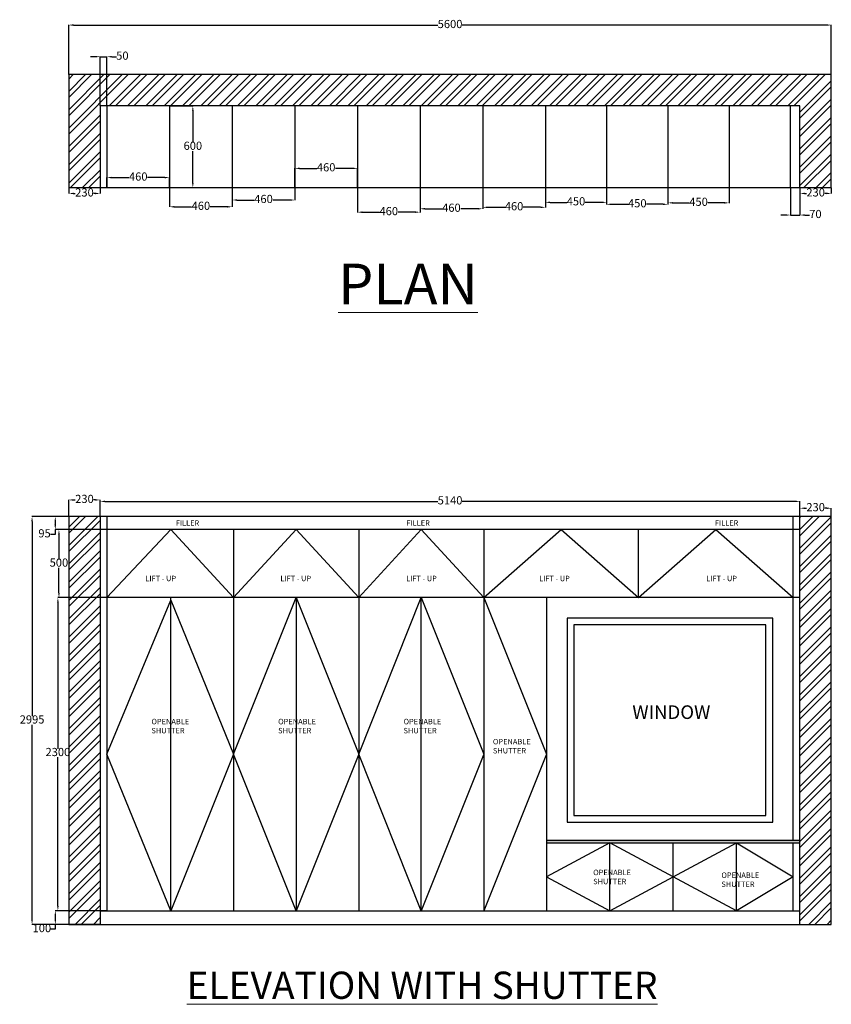
# Model space of a CAD drawing. Units: millimetres. Extents: x 1304 to 14372, y 283 to 7516.
# Tile 4 of 4: x 8411 to 14372, y 283 to 7516. Entities that reach past the tile are written whole.
import ezdxf

# ---------------------------------------------------------------- set-up
doc = ezdxf.new("R2010")
doc.units = ezdxf.units.MM
doc.layers.get('Defpoints').update_dxf_attribs({"color": 2})
for name, color, linetype, lineweight in [('A-ANNO-DIMS', 2, 'Continuous', 18), ('A-ANNO-TEXT', 3, 'Continuous', 18), ('A-FURN', 7, 'Continuous', 25), ('A-FURN-PATT', 8, 'Continuous', 13)]:
    doc.layers.add(name, color=color, linetype=linetype, lineweight=lineweight)
doc.styles.get("Standard").update_dxf_attribs({"font": 'arial.ttf'})
doc.dimstyles.new('ISO-25', dxfattribs={"dimtxt": 60, "dimasz": 35, "dimexe": 1.25, "dimexo": 0.625, "dimtad": 0, "dimtih": 1, "dimtoh": 1, "dimtxsty": 'Standard', "dimcen": 2.5, "dimclrd": 1, "dimclre": 3, "dimadec": 0, "dimazin": 0, "dimtfac": 1, "dimtmove": 0, "dimatfit": 3, "dimfxl": 1, "dimarcsym": 0})

# ---------------------------------------------------------------- blocks, each defined once
blk = doc.blocks.new('*D46')
at = {"layer": 'A-ANNO-DIMS', "color": 0, "lineweight": -2, "transparency": 16777216}
for p, q in [((8771.4, 3865.3), (8500.9, 3865.3)), ((8502.2, 3830.3), (8502.2, 2399)), ((8502.2, 905.3), (8502.2, 2336.5)), ((8771.4, 870.3), (8500.9, 870.3))]:
    blk.add_line(p, q, dxfattribs=at)
at = {"layer": 'A-ANNO-DIMS', "color": 0, "transparency": 16777216}
for points in [[(8496.3, 3830.3), (8508, 3830.3), (8502.2, 3865.3)], [(8496.3, 905.3), (8508, 905.3), (8502.2, 870.3)]]:
    blk.add_solid(points, dxfattribs=at)
at = {"layer": 'Defpoints', "color": 0, "transparency": 16777216}
for p in [(8772, 3865.3), (8502.2, 870.3), (8772, 870.3)]:
    blk.add_point(p, dxfattribs=at)
at = {"layer": 'A-ANNO-DIMS', "color": 0, "transparency": 16777216, "insert": (8502.2, 2367.8), "char_height": 60, "attachment_point": 5}
blk.add_mtext('2995', dxfattribs=at)
blk = doc.blocks.new('*D47')
at = {"layer": 'A-ANNO-DIMS', "color": 0, "lineweight": -2, "transparency": 16777216}
for p, q in [((9001.4, 3865.3), (8671.3, 3865.3)), ((9001.4, 3770.3), (8671.3, 3770.3)), ((8672.5, 3830.3), (8672.5, 3805.3)), ((8672.5, 3770.3), (8672.5, 3735.3)), ((8672.5, 3735.3), (8637.5, 3735.3))]:
    blk.add_line(p, q, dxfattribs=at)
at = {"layer": 'A-ANNO-DIMS', "color": 0, "transparency": 16777216}
for points in [[(8666.7, 3830.3), (8678.4, 3830.3), (8672.5, 3865.3)], [(8666.7, 3805.3), (8678.4, 3805.3), (8672.5, 3770.3)]]:
    blk.add_solid(points, dxfattribs=at)
at = {"layer": 'Defpoints', "color": 0, "transparency": 16777216}
for p in [(9002, 3865.3), (8672.5, 3770.3), (9002, 3770.3)]:
    blk.add_point(p, dxfattribs=at)
at = {"layer": 'A-ANNO-DIMS', "color": 0, "transparency": 16777216, "insert": (8593.7, 3735.3), "char_height": 60, "attachment_point": 5}
blk.add_mtext('95', dxfattribs=at)
blk = doc.blocks.new('*D48')
at = {"layer": 'A-ANNO-DIMS', "color": 0, "lineweight": -2, "transparency": 16777216}
for p, q in [((9051.4, 3770.3), (8698.2, 3770.3)), ((8699.5, 3735.3), (8699.5, 3551.5)), ((8699.5, 3305.3), (8699.5, 3489)), ((9051.4, 3270.3), (8698.2, 3270.3))]:
    blk.add_line(p, q, dxfattribs=at)
at = {"layer": 'A-ANNO-DIMS', "color": 0, "transparency": 16777216}
for points in [[(8693.6, 3735.3), (8705.3, 3735.3), (8699.5, 3770.3)], [(8693.6, 3305.3), (8705.3, 3305.3), (8699.5, 3270.3)]]:
    blk.add_solid(points, dxfattribs=at)
at = {"layer": 'Defpoints', "color": 0, "transparency": 16777216}
for p in [(9052, 3770.3), (8699.5, 3270.3), (9052, 3270.3)]:
    blk.add_point(p, dxfattribs=at)
at = {"layer": 'A-ANNO-DIMS', "color": 0, "transparency": 16777216, "insert": (8699.5, 3520.3), "char_height": 60, "attachment_point": 5}
blk.add_mtext('500', dxfattribs=at)
blk = doc.blocks.new('*D49')
at = {"layer": 'A-ANNO-DIMS', "color": 0, "lineweight": -2, "transparency": 16777216}
for p, q in [((9001.4, 970.3), (8671.7, 970.3)), ((9001.4, 870.3), (8671.7, 870.3)), ((8673, 935.3), (8673, 905.3)), ((8673, 870.3), (8673, 835.3)), ((8673, 835.3), (8638, 835.3))]:
    blk.add_line(p, q, dxfattribs=at)
at = {"layer": 'A-ANNO-DIMS', "color": 0, "transparency": 16777216}
for points in [[(8667.1, 935.3), (8678.8, 935.3), (8673, 970.3)], [(8667.1, 905.3), (8678.8, 905.3), (8673, 870.3)]]:
    blk.add_solid(points, dxfattribs=at)
at = {"layer": 'Defpoints', "color": 0, "transparency": 16777216}
for p in [(9002, 970.3), (8673, 870.3), (9002, 870.3)]:
    blk.add_point(p, dxfattribs=at)
at = {"layer": 'A-ANNO-DIMS', "color": 0, "transparency": 16777216, "insert": (8574, 835.3), "char_height": 60, "attachment_point": 5}
blk.add_mtext('100', dxfattribs=at)
blk = doc.blocks.new('*D50')
at = {"layer": 'A-ANNO-DIMS', "color": 0, "lineweight": -2, "transparency": 16777216}
for p, q in [((9051.4, 3270.3), (8690.6, 3270.3)), ((8691.9, 3235.3), (8691.9, 2160)), ((8691.9, 1005.3), (8691.9, 2097.5)), ((9051.4, 970.3), (8690.6, 970.3))]:
    blk.add_line(p, q, dxfattribs=at)
at = {"layer": 'A-ANNO-DIMS', "color": 0, "transparency": 16777216}
for points in [[(8686.1, 3235.3), (8697.7, 3235.3), (8691.9, 3270.3)], [(8686.1, 1005.3), (8697.7, 1005.3), (8691.9, 970.3)]]:
    blk.add_solid(points, dxfattribs=at)
at = {"layer": 'Defpoints', "color": 0, "transparency": 16777216}
for p in [(9052, 3270.3), (8691.9, 970.3), (9052, 970.3)]:
    blk.add_point(p, dxfattribs=at)
at = {"layer": 'A-ANNO-DIMS', "color": 0, "transparency": 16777216, "insert": (8691.9, 2128.8), "char_height": 60, "attachment_point": 5}
blk.add_mtext('2300', dxfattribs=at)
blk = doc.blocks.new('*D51')
at = {"layer": 'A-ANNO-DIMS', "color": 0, "lineweight": -2, "transparency": 16777216}
for p, q in [((8772, 3865.9), (8772, 3989.4)), ((8807, 3988.1), (8819.7, 3988.1)), ((8967, 3988.1), (8954.3, 3988.1)), ((9002, 3865.9), (9002, 3989.4))]:
    blk.add_line(p, q, dxfattribs=at)
at = {"layer": 'A-ANNO-DIMS', "color": 0, "transparency": 16777216}
for points in [[(8807, 3993.9), (8807, 3982.3), (8772, 3988.1)], [(8967, 3993.9), (8967, 3982.3), (9002, 3988.1)]]:
    blk.add_solid(points, dxfattribs=at)
at = {"layer": 'Defpoints', "color": 0, "transparency": 16777216}
for p in [(9002, 3988.1), (8772, 3865.3), (9002, 3865.3)]:
    blk.add_point(p, dxfattribs=at)
at = {"layer": 'A-ANNO-DIMS', "color": 0, "transparency": 16777216, "insert": (8887, 3988.1), "char_height": 60, "attachment_point": 5}
blk.add_mtext('230', dxfattribs=at)
blk = doc.blocks.new('*D52')
at = {"layer": 'A-ANNO-DIMS', "color": 0, "lineweight": -2, "transparency": 16777216}
for p, q in [((14142, 3865.9), (14142, 3928.7)), ((14177, 3927.4), (14189.7, 3927.4)), ((14337, 3927.4), (14324.3, 3927.4)), ((14372, 3865.9), (14372, 3928.7))]:
    blk.add_line(p, q, dxfattribs=at)
at = {"layer": 'A-ANNO-DIMS', "color": 0, "transparency": 16777216}
for points in [[(14177, 3933.2), (14177, 3921.6), (14142, 3927.4)], [(14337, 3933.2), (14337, 3921.6), (14372, 3927.4)]]:
    blk.add_solid(points, dxfattribs=at)
at = {"layer": 'Defpoints', "color": 0, "transparency": 16777216}
for p in [(14372, 3927.4), (14142, 3865.3), (14372, 3865.3)]:
    blk.add_point(p, dxfattribs=at)
at = {"layer": 'A-ANNO-DIMS', "color": 0, "transparency": 16777216, "insert": (14257, 3927.4), "char_height": 60, "attachment_point": 5}
blk.add_mtext('230', dxfattribs=at)
blk = doc.blocks.new('*D53')
at = {"layer": 'A-ANNO-DIMS', "color": 0, "lineweight": -2, "transparency": 16777216}
for p, q in [((9002, 3865.9), (9002, 3978.7)), ((14142, 3865.9), (14142, 3978.7)), ((9037, 3977.4), (11481.9, 3977.4)), ((14107, 3977.4), (11662.1, 3977.4))]:
    blk.add_line(p, q, dxfattribs=at)
at = {"layer": 'A-ANNO-DIMS', "color": 0, "transparency": 16777216}
for points in [[(9037, 3983.2), (9037, 3971.6), (9002, 3977.4)], [(14107, 3983.2), (14107, 3971.6), (14142, 3977.4)]]:
    blk.add_solid(points, dxfattribs=at)
at = {"layer": 'Defpoints', "color": 0, "transparency": 16777216}
for p in [(14142, 3977.4), (9002, 3865.3), (14142, 3865.3)]:
    blk.add_point(p, dxfattribs=at)
at = {"layer": 'A-ANNO-DIMS', "color": 0, "transparency": 16777216, "insert": (11572, 3977.4), "char_height": 60, "attachment_point": 5}
blk.add_mtext('5140', dxfattribs=at)
blk = doc.blocks.new('*D54')
at = {"layer": 'A-ANNO-DIMS', "color": 0, "lineweight": -2, "transparency": 16777216}
for p, q in [((8772, 6281.6), (8772, 6238)), ((8807, 6239.3), (8819.7, 6239.3)), ((8967, 6239.3), (8954.3, 6239.3)), ((9002, 6281.6), (9002, 6238))]:
    blk.add_line(p, q, dxfattribs=at)
at = {"layer": 'A-ANNO-DIMS', "color": 0, "transparency": 16777216}
for points in [[(8807, 6245.1), (8807, 6233.4), (8772, 6239.3)], [(8967, 6245.1), (8967, 6233.4), (9002, 6239.3)]]:
    blk.add_solid(points, dxfattribs=at)
at = {"layer": 'Defpoints', "color": 0, "transparency": 16777216}
for p in [(8772, 6282.2), (9002, 6282.2), (9002, 6239.3)]:
    blk.add_point(p, dxfattribs=at)
at = {"layer": 'A-ANNO-DIMS', "color": 0, "transparency": 16777216, "insert": (8887, 6239.3), "char_height": 60, "attachment_point": 5}
blk.add_mtext('230', dxfattribs=at)
blk = doc.blocks.new('*D55')
at = {"layer": 'A-ANNO-DIMS', "color": 0, "lineweight": -2, "transparency": 16777216}
for p, q in [((8967, 7244), (8932, 7244)), ((9002, 6882.8), (9002, 7245.2)), ((9002, 7244), (9052, 7244)), ((9052, 6882.8), (9052, 7245.2)), ((9087, 7244), (9122, 7244))]:
    blk.add_line(p, q, dxfattribs=at)
at = {"layer": 'A-ANNO-DIMS', "color": 0, "transparency": 16777216}
for points in [[(8967, 7249.8), (8967, 7238.2), (9002, 7244)], [(9087, 7249.8), (9087, 7238.2), (9052, 7244)]]:
    blk.add_solid(points, dxfattribs=at)
at = {"layer": 'Defpoints', "color": 0, "transparency": 16777216}
for p in [(9052, 7244), (9002, 6882.2), (9052, 6882.2)]:
    blk.add_point(p, dxfattribs=at)
at = {"layer": 'A-ANNO-DIMS', "color": 0, "transparency": 16777216, "insert": (9165.5, 7244), "char_height": 60, "attachment_point": 5}
blk.add_mtext('50', dxfattribs=at)
blk = doc.blocks.new('*D56')
at = {"layer": 'A-ANNO-DIMS', "color": 0, "lineweight": -2, "transparency": 16777216}
for p, q in [((9052, 6282.8), (9052, 6357.4)), ((9087, 6356.1), (9214, 6356.1)), ((9477, 6356.1), (9350, 6356.1)), ((9512, 6282.8), (9512, 6357.4))]:
    blk.add_line(p, q, dxfattribs=at)
at = {"layer": 'A-ANNO-DIMS', "color": 0, "transparency": 16777216}
for points in [[(9087, 6361.9), (9087, 6350.3), (9052, 6356.1)], [(9477, 6361.9), (9477, 6350.3), (9512, 6356.1)]]:
    blk.add_solid(points, dxfattribs=at)
at = {"layer": 'Defpoints', "color": 0, "transparency": 16777216}
for p in [(9512, 6356.1), (9052, 6282.2), (9512, 6282.2)]:
    blk.add_point(p, dxfattribs=at)
at = {"layer": 'A-ANNO-DIMS', "color": 0, "transparency": 16777216, "insert": (9282, 6356.1), "char_height": 60, "attachment_point": 5}
blk.add_mtext('460', dxfattribs=at)
blk = doc.blocks.new('*D57')
at = {"layer": 'A-ANNO-DIMS', "color": 0, "lineweight": -2, "transparency": 16777216}
for p, q in [((9512, 6281.6), (9512, 6140.1)), ((9972, 6281.6), (9972, 6140.1)), ((9547, 6141.3), (9674, 6141.3)), ((9937, 6141.3), (9810, 6141.3))]:
    blk.add_line(p, q, dxfattribs=at)
at = {"layer": 'A-ANNO-DIMS', "color": 0, "transparency": 16777216}
for points in [[(9547, 6147.2), (9547, 6135.5), (9512, 6141.3)], [(9937, 6147.2), (9937, 6135.5), (9972, 6141.3)]]:
    blk.add_solid(points, dxfattribs=at)
at = {"layer": 'Defpoints', "color": 0, "transparency": 16777216}
for p in [(9512, 6282.2), (9972, 6282.2), (9972, 6141.3)]:
    blk.add_point(p, dxfattribs=at)
at = {"layer": 'A-ANNO-DIMS', "color": 0, "transparency": 16777216, "insert": (9742, 6141.3), "char_height": 60, "attachment_point": 5}
blk.add_mtext('460', dxfattribs=at)
blk = doc.blocks.new('*D58')
at = {"layer": 'A-ANNO-DIMS', "color": 0, "lineweight": -2, "transparency": 16777216}
for p, q in [((9972, 6281.6), (9972, 6190.2)), ((10432, 6281.6), (10432, 6190.2)), ((10007, 6191.4), (10134, 6191.4)), ((10397, 6191.4), (10270, 6191.4))]:
    blk.add_line(p, q, dxfattribs=at)
at = {"layer": 'A-ANNO-DIMS', "color": 0, "transparency": 16777216}
for points in [[(10007, 6197.2), (10007, 6185.6), (9972, 6191.4)], [(10397, 6197.2), (10397, 6185.6), (10432, 6191.4)]]:
    blk.add_solid(points, dxfattribs=at)
at = {"layer": 'Defpoints', "color": 0, "transparency": 16777216}
for p in [(9972, 6282.2), (10432, 6282.2), (10432, 6191.4)]:
    blk.add_point(p, dxfattribs=at)
at = {"layer": 'A-ANNO-DIMS', "color": 0, "transparency": 16777216, "insert": (10202, 6191.4), "char_height": 60, "attachment_point": 5}
blk.add_mtext('460', dxfattribs=at)
blk = doc.blocks.new('*D59')
at = {"layer": 'A-ANNO-DIMS', "color": 0, "lineweight": -2, "transparency": 16777216}
for p, q in [((10432, 6282.8), (10432, 6425.1)), ((10467, 6423.9), (10594, 6423.9)), ((10857, 6423.9), (10730, 6423.9)), ((10892, 6282.8), (10892, 6425.1))]:
    blk.add_line(p, q, dxfattribs=at)
at = {"layer": 'A-ANNO-DIMS', "color": 0, "transparency": 16777216}
for points in [[(10467, 6429.7), (10467, 6418), (10432, 6423.9)], [(10857, 6429.7), (10857, 6418), (10892, 6423.9)]]:
    blk.add_solid(points, dxfattribs=at)
at = {"layer": 'Defpoints', "color": 0, "transparency": 16777216}
for p in [(10892, 6423.9), (10432, 6282.2), (10892, 6282.2)]:
    blk.add_point(p, dxfattribs=at)
at = {"layer": 'A-ANNO-DIMS', "color": 0, "transparency": 16777216, "insert": (10662, 6423.9), "char_height": 60, "attachment_point": 5}
blk.add_mtext('460', dxfattribs=at)
blk = doc.blocks.new('*D60')
at = {"layer": 'A-ANNO-DIMS', "color": 0, "lineweight": -2, "transparency": 16777216}
for p, q in [((10892, 6281.6), (10892, 6100.7)), ((11352, 6281.6), (11352, 6100.7)), ((10927, 6102), (11054, 6102)), ((11317, 6102), (11190, 6102))]:
    blk.add_line(p, q, dxfattribs=at)
at = {"layer": 'A-ANNO-DIMS', "color": 0, "transparency": 16777216}
for points in [[(10927, 6107.8), (10927, 6096.2), (10892, 6102)], [(11317, 6107.8), (11317, 6096.2), (11352, 6102)]]:
    blk.add_solid(points, dxfattribs=at)
at = {"layer": 'Defpoints', "color": 0, "transparency": 16777216}
for p in [(10892, 6282.2), (11352, 6282.2), (11352, 6102)]:
    blk.add_point(p, dxfattribs=at)
at = {"layer": 'A-ANNO-DIMS', "color": 0, "transparency": 16777216, "insert": (11122, 6102), "char_height": 60, "attachment_point": 5}
blk.add_mtext('460', dxfattribs=at)
blk = doc.blocks.new('*D61')
at = {"layer": 'A-ANNO-DIMS', "color": 0, "lineweight": -2, "transparency": 16777216}
for p, q in [((11352, 6281.6), (11352, 6125.8)), ((11812, 6281.6), (11812, 6125.8)), ((11387, 6127), (11514, 6127)), ((11777, 6127), (11650, 6127))]:
    blk.add_line(p, q, dxfattribs=at)
at = {"layer": 'A-ANNO-DIMS', "color": 0, "transparency": 16777216}
for points in [[(11387, 6132.9), (11387, 6121.2), (11352, 6127)], [(11777, 6132.9), (11777, 6121.2), (11812, 6127)]]:
    blk.add_solid(points, dxfattribs=at)
at = {"layer": 'Defpoints', "color": 0, "transparency": 16777216}
for p in [(11352, 6282.2), (11812, 6282.2), (11812, 6127)]:
    blk.add_point(p, dxfattribs=at)
at = {"layer": 'A-ANNO-DIMS', "color": 0, "transparency": 16777216, "insert": (11582, 6127), "char_height": 60, "attachment_point": 5}
blk.add_mtext('460', dxfattribs=at)
blk = doc.blocks.new('*D62')
at = {"layer": 'A-ANNO-DIMS', "color": 0, "lineweight": -2, "transparency": 16777216}
for p, q in [((11812, 6281.6), (11812, 6136.5)), ((12272, 6281.6), (12272, 6136.5)), ((11847, 6137.8), (11974, 6137.8)), ((12237, 6137.8), (12110, 6137.8))]:
    blk.add_line(p, q, dxfattribs=at)
at = {"layer": 'A-ANNO-DIMS', "color": 0, "transparency": 16777216}
for points in [[(11847, 6143.6), (11847, 6131.9), (11812, 6137.8)], [(12237, 6143.6), (12237, 6131.9), (12272, 6137.8)]]:
    blk.add_solid(points, dxfattribs=at)
at = {"layer": 'Defpoints', "color": 0, "transparency": 16777216}
for p in [(11812, 6282.2), (12272, 6282.2), (12272, 6137.8)]:
    blk.add_point(p, dxfattribs=at)
at = {"layer": 'A-ANNO-DIMS', "color": 0, "transparency": 16777216, "insert": (12042, 6137.8), "char_height": 60, "attachment_point": 5}
blk.add_mtext('460', dxfattribs=at)
blk = doc.blocks.new('*D63')
at = {"layer": 'A-ANNO-DIMS', "color": 0, "lineweight": -2, "transparency": 16777216}
for p, q in [((12272, 6281.6), (12272, 6172.9)), ((12722, 6281.6), (12722, 6172.9)), ((12307, 6174.1), (12429, 6174.1)), ((12687, 6174.1), (12565, 6174.1))]:
    blk.add_line(p, q, dxfattribs=at)
at = {"layer": 'A-ANNO-DIMS', "color": 0, "transparency": 16777216}
for points in [[(12307, 6180), (12307, 6168.3), (12272, 6174.1)], [(12687, 6180), (12687, 6168.3), (12722, 6174.1)]]:
    blk.add_solid(points, dxfattribs=at)
at = {"layer": 'Defpoints', "color": 0, "transparency": 16777216}
for p in [(12272, 6282.2), (12722, 6282.2), (12722, 6174.1)]:
    blk.add_point(p, dxfattribs=at)
at = {"layer": 'A-ANNO-DIMS', "color": 0, "transparency": 16777216, "insert": (12497, 6174.1), "char_height": 60, "attachment_point": 5}
blk.add_mtext('450', dxfattribs=at)
blk = doc.blocks.new('*D64')
at = {"layer": 'A-ANNO-DIMS', "color": 0, "lineweight": -2, "transparency": 16777216}
for p, q in [((12722, 6281.6), (12722, 6158.5)), ((13172, 6281.6), (13172, 6158.5)), ((12757, 6159.8), (12879, 6159.8)), ((13137, 6159.8), (13015, 6159.8))]:
    blk.add_line(p, q, dxfattribs=at)
at = {"layer": 'A-ANNO-DIMS', "color": 0, "transparency": 16777216}
for points in [[(12757, 6165.6), (12757, 6153.9), (12722, 6159.8)], [(13137, 6165.6), (13137, 6153.9), (13172, 6159.8)]]:
    blk.add_solid(points, dxfattribs=at)
at = {"layer": 'Defpoints', "color": 0, "transparency": 16777216}
for p in [(12722, 6282.2), (13172, 6282.2), (13172, 6159.8)]:
    blk.add_point(p, dxfattribs=at)
at = {"layer": 'A-ANNO-DIMS', "color": 0, "transparency": 16777216, "insert": (12947, 6159.8), "char_height": 60, "attachment_point": 5}
blk.add_mtext('450', dxfattribs=at)
blk = doc.blocks.new('*D65')
at = {"layer": 'A-ANNO-DIMS', "color": 0, "lineweight": -2, "transparency": 16777216}
for p, q in [((13172, 6281.6), (13172, 6169.3)), ((13622, 6281.6), (13622, 6169.3)), ((13207, 6170.5), (13329, 6170.5)), ((13587, 6170.5), (13465, 6170.5))]:
    blk.add_line(p, q, dxfattribs=at)
at = {"layer": 'A-ANNO-DIMS', "color": 0, "transparency": 16777216}
for points in [[(13207, 6176.4), (13207, 6164.7), (13172, 6170.5)], [(13587, 6176.4), (13587, 6164.7), (13622, 6170.5)]]:
    blk.add_solid(points, dxfattribs=at)
at = {"layer": 'Defpoints', "color": 0, "transparency": 16777216}
for p in [(13172, 6282.2), (13622, 6282.2), (13622, 6170.5)]:
    blk.add_point(p, dxfattribs=at)
at = {"layer": 'A-ANNO-DIMS', "color": 0, "transparency": 16777216, "insert": (13397, 6170.5), "char_height": 60, "attachment_point": 5}
blk.add_mtext('450', dxfattribs=at)
blk = doc.blocks.new('*D66')
at = {"layer": 'A-ANNO-DIMS', "color": 0, "lineweight": -2, "transparency": 16777216}
for p, q in [((14142, 6281.6), (14142, 6238.3)), ((14177, 6239.6), (14189.7, 6239.6)), ((14337, 6239.6), (14324.3, 6239.6)), ((14372, 6281.6), (14372, 6238.3))]:
    blk.add_line(p, q, dxfattribs=at)
at = {"layer": 'A-ANNO-DIMS', "color": 0, "transparency": 16777216}
for points in [[(14177, 6245.4), (14177, 6233.7), (14142, 6239.6)], [(14337, 6245.4), (14337, 6233.7), (14372, 6239.6)]]:
    blk.add_solid(points, dxfattribs=at)
at = {"layer": 'Defpoints', "color": 0, "transparency": 16777216}
for p in [(14142, 6282.2), (14142, 6239.6), (14372, 6282.2)]:
    blk.add_point(p, dxfattribs=at)
at = {"layer": 'A-ANNO-DIMS', "color": 0, "transparency": 16777216, "insert": (14257, 6239.6), "char_height": 60, "attachment_point": 5}
blk.add_mtext('230', dxfattribs=at)
blk = doc.blocks.new('*D67')
at = {"layer": 'A-ANNO-DIMS', "color": 0, "lineweight": -2, "transparency": 16777216}
for p, q in [((14072, 6281.6), (14072, 6079.6)), ((14142, 6281.6), (14142, 6079.6)), ((14037, 6080.9), (14002, 6080.9)), ((14072, 6080.9), (14142, 6080.9)), ((14177, 6080.9), (14212, 6080.9))]:
    blk.add_line(p, q, dxfattribs=at)
at = {"layer": 'A-ANNO-DIMS', "color": 0, "transparency": 16777216}
for points in [[(14037, 6086.7), (14037, 6075), (14072, 6080.9)], [(14177, 6086.7), (14177, 6075), (14142, 6080.9)]]:
    blk.add_solid(points, dxfattribs=at)
at = {"layer": 'Defpoints', "color": 0, "transparency": 16777216}
for p in [(14072, 6282.2), (14142, 6282.2), (14142, 6080.9)]:
    blk.add_point(p, dxfattribs=at)
at = {"layer": 'A-ANNO-DIMS', "color": 0, "transparency": 16777216, "insert": (14255.2, 6080.9), "char_height": 60, "attachment_point": 5}
blk.add_mtext('70', dxfattribs=at)
blk = doc.blocks.new('*D68')
at = {"layer": 'A-ANNO-DIMS', "color": 0, "lineweight": -2, "transparency": 16777216}
for p, q in [((8772, 7112.8), (8772, 7477.8)), ((8807, 7476.5), (11481.9, 7476.5)), ((14337, 7476.5), (11662.1, 7476.5)), ((14372, 7112.8), (14372, 7477.8))]:
    blk.add_line(p, q, dxfattribs=at)
at = {"layer": 'A-ANNO-DIMS', "color": 0, "transparency": 16777216}
for points in [[(8807, 7482.4), (8807, 7470.7), (8772, 7476.5)], [(14337, 7482.4), (14337, 7470.7), (14372, 7476.5)]]:
    blk.add_solid(points, dxfattribs=at)
at = {"layer": 'Defpoints', "color": 0, "transparency": 16777216}
for p in [(14372, 7476.5), (8772, 7112.2), (14372, 7112.2)]:
    blk.add_point(p, dxfattribs=at)
at = {"layer": 'A-ANNO-DIMS', "color": 0, "transparency": 16777216, "insert": (11572, 7476.5), "char_height": 60, "attachment_point": 5}
blk.add_mtext('5600', dxfattribs=at)
blk = doc.blocks.new('*D69')
at = {"layer": 'A-ANNO-DIMS', "color": 0, "lineweight": -2, "transparency": 16777216}
for p, q in [((9512.6, 6882.2), (9684.3, 6882.2)), ((9683, 6847.2), (9683, 6613.5)), ((9683, 6317.2), (9683, 6551)), ((9512.6, 6282.2), (9684.3, 6282.2))]:
    blk.add_line(p, q, dxfattribs=at)
at = {"layer": 'A-ANNO-DIMS', "color": 0, "transparency": 16777216}
for points in [[(9677.2, 6847.2), (9688.8, 6847.2), (9683, 6882.2)], [(9677.2, 6317.2), (9688.8, 6317.2), (9683, 6282.2)]]:
    blk.add_solid(points, dxfattribs=at)
at = {"layer": 'Defpoints', "color": 0, "transparency": 16777216}
for p in [(9512, 6882.2), (9512, 6282.2), (9683, 6282.2)]:
    blk.add_point(p, dxfattribs=at)
at = {"layer": 'A-ANNO-DIMS', "color": 0, "transparency": 16777216, "insert": (9683, 6582.2), "char_height": 60, "attachment_point": 5}
blk.add_mtext('600', dxfattribs=at)

msp = doc.modelspace()

# ---------------------------------------------------------------- hatches: boundary and pattern name
at = {"layer": 'A-FURN-PATT'}
h = msp.add_hatch(dxfattribs=at)
h.set_pattern_fill('ANSI32', color=256, scale=10)
h.set_pattern_definition([(45, (0, 1046.14), (-67.3519, 67.3519), []), (45, (44.9, 1046.14), (-67.3519, 67.3519), [])])
h.paths.add_polyline_path([(8771.982, 6282.215), (9001.982, 6282.215), (9001.982, 6882.215), (14141.982, 6882.215), (14141.982, 6282.215), (14371.982, 6282.215), (14371.982, 7112.215), (8771.982, 7112.215)])
h = msp.add_hatch(dxfattribs=at)
h.set_pattern_fill('ANSI32', color=256, scale=10)
h.paths.add_polyline_path([(9001.982, 3865.285), (8771.982, 3865.285), (8771.982, 870.285), (9001.982, 870.285)])
h.paths.add_polyline_path([(14371.982, 3865.285), (14141.982, 3865.285), (14141.982, 870.285), (14371.982, 870.285)])
h = msp.add_hatch(color=256, dxfattribs=at)
h.dxf.hatch_style = 1
h.paths.add_polyline_path([(14091.982, 1488.285), (12280.982, 1488.285), (12280.982, 1470.285), (14091.982, 1470.285)])
h = msp.add_hatch(color=256, dxfattribs=at)
h.dxf.hatch_style = 1
h.paths.add_polyline_path([(14141.982, 1488.285), (12280.982, 1488.285), (12280.982, 1470.285), (14141.982, 1470.285)])

# ---------------------------------------------------------------- linework, layer by layer
at = {"layer": 'A-FURN'}
for p, q in [((14371.982, 7112.215), (8771.982, 7112.215)), ((8771.982, 7112.215), (8771.982, 6282.215)), ((14371.982, 6282.215), (14371.982, 7112.215)), ((9001.982, 6882.215), (9001.982, 6282.215)), ((14141.982, 6882.215), (9001.982, 6882.215)), ((9051.982, 6882.215), (9051.982, 6282.215)), ((9511.982, 6882.215), (9511.982, 6282.215)), ((9971.982, 6882.215), (9971.982, 6282.215)), ((10431.982, 6882.215), (10431.982, 6282.215)), ((10891.982, 6882.215), (10891.982, 6282.215)), ((11351.982, 6882.215), (11351.982, 6282.215)), ((11811.982, 6882.215), (11811.982, 6282.215)), ((12271.982, 6882.215), (12271.982, 6282.215)), ((12721.982, 6882.215), (12721.982, 6282.215)), ((13171.982, 6882.215), (13171.982, 6282.215)), ((13621.982, 6882.215), (13621.982, 6282.215)), ((14071.982, 6282.215), (14071.982, 6882.215)), ((14141.982, 6282.215), (14141.982, 6882.215)), ((8771.982, 6282.215), (14371.982, 6282.215)), ((14371.982, 3865.285), (8771.982, 3865.285)), ((8771.982, 3865.285), (8771.982, 870.285)), ((9001.982, 3865.285), (9001.982, 870.285)), ((9051.982, 3865.285), (9051.982, 970.285)), ((14091.982, 3270.285), (14091.982, 3865.285)), ((14141.982, 870.285), (14141.982, 3865.285)), ((14371.982, 870.285), (14371.982, 3865.285)), ((14141.982, 3770.285), (9001.982, 3770.285)), ((9051.982, 3270.285), (9520.982, 3770.285)), ((9520.982, 3770.285), (9980.982, 3270.285)), ((9980.982, 3770.285), (9980.982, 970.285)), ((9980.982, 3270.285), (10440.982, 3770.285)), ((10440.982, 3770.285), (10900.982, 3270.285)), ((10900.982, 3770.285), (10900.982, 970.285)), ((10900.982, 3270.285), (11360.982, 3770.285)), ((11360.982, 3770.285), (11820.982, 3270.285)), ((11820.982, 3770.285), (11820.982, 970.285)), ((11820.982, 3270.285), (12388.732, 3770.285)), ((12388.732, 3770.285), (12956.482, 3270.285)), ((12956.482, 3270.285), (12956.482, 3770.285)), ((12956.482, 3270.285), (13524.232, 3770.285)), ((13524.232, 3770.285), (14091.982, 3270.285)), ((12280.982, 3270.285), (9001.982, 3270.285)), ((9520.982, 970.285), (9520.982, 3270.285)), ((9980.982, 3270.285), (9980.982, 3270.285)), ((9980.982, 2120.285), (10440.982, 3270.285)), ((10440.982, 3270.285), (10440.982, 970.285)), ((10440.982, 3270.285), (10900.982, 2120.285)), ((10900.982, 2120.285), (11360.982, 3270.285)), ((11360.982, 970.285), (11360.982, 3270.285)), ((11360.982, 3270.285), (11820.982, 2120.285)), ((11820.982, 3270.285), (12280.982, 2120.285)), ((14091.982, 3270.285), (12280.982, 3270.285)), ((12280.982, 3270.285), (12280.982, 1470.285)), ((14141.982, 3270.285), (14091.982, 3270.285)), ((14091.982, 1488.285), (14091.982, 3270.285)), ((9051.982, 2120.285), (9520.982, 3252.551)), ((9520.982, 3252.551), (9980.982, 2120.285)), ((9520.982, 970.285), (9051.982, 2120.285)), ((9980.982, 2120.285), (9520.982, 970.285)), ((10440.982, 970.285), (9980.982, 2120.285)), ((10900.982, 2120.285), (10440.982, 970.285)), ((11360.982, 970.285), (10900.982, 2120.285)), ((11820.982, 2120.285), (11360.982, 970.285)), ((12280.982, 2120.285), (11820.982, 970.285)), ((12280.982, 1488.285), (14141.982, 1488.285)), ((12746.232, 1470.285), (12280.982, 1220.285)), ((12280.982, 1470.285), (12280.982, 970.285)), ((12280.982, 1470.285), (14141.982, 1470.285)), ((12746.232, 970.285), (12746.232, 1470.285)), ((13211.482, 1220.285), (12746.232, 1470.285)), ((13211.482, 970.285), (13211.482, 1470.285)), ((13211.482, 1220.285), (13676.732, 1470.285)), ((13676.732, 970.285), (13676.732, 1470.285)), ((13676.732, 1470.285), (14091.982, 1220.285)), ((14091.982, 970.285), (14091.982, 1470.285)), ((12280.982, 1220.285), (12746.232, 970.285)), ((12746.232, 970.285), (13211.482, 1220.285)), ((13676.732, 970.285), (13211.482, 1220.285)), ((14091.982, 1220.285), (13676.732, 970.285)), ((9001.982, 970.285), (12280.982, 970.285)), ((12280.982, 970.285), (13211.482, 970.285)), ((13211.482, 970.285), (14141.982, 970.285)), ((8771.982, 870.285), (14371.982, 870.285))]:
    msp.add_line(p, q, dxfattribs=at)
for points in [[(13941.982, 1620.285), (13941.982, 3120.285), (12430.982, 3120.285), (12430.982, 1620.285)], [(13891.982, 1670.285), (13891.982, 3070.285), (12480.982, 3070.285), (12480.982, 1670.285)]]:
    msp.add_lwpolyline(points, close=True, dxfattribs=at)

# ---------------------------------------------------------------- texts
at = {"layer": 'A-ANNO-TEXT', "attachment_point": 1}
for s, width, gutter_width, heights, insert, char_height in [('{\\H0.08377x;\\P\\H11.93779x;\\LPLAN}', 2990.54211, 17906.681, [0], (10749.837, 5765.834), 300), ('FILLER', 605.86509, 50, [0], (9557.521, 3838.722), 40), ('FILLER', 605.86509, 50, [0], (11251.367, 3838.722), 40), ('FILLER', 605.86509, 50, [0], (13517.256, 3838.722), 40), ('LIFT - UP', 605.86509, 50, [0], (9334.268, 3431.393), 40), ('LIFT - UP', 605.86509, 50, [0], (10326.099, 3431.393), 40), ('LIFT - UP', 605.86509, 50, [0], (11249.526, 3431.393), 40), ('LIFT - UP', 605.86509, 50, [0], (12226.156, 3431.393), 40), ('LIFT - UP', 605.86509, 50, [0], (13453.853, 3431.393), 40), ('WINDOW', 605.86509, 50, [103.479], (12910.645, 2479.331), 100), ('OPENABLE SHUTTER', 452.88831, 50, [0], (9378.774, 2380.165), 40), ('OPENABLE SHUTTER', 452.88831, 50, [0], (10309.637, 2380.165), 40), ('OPENABLE SHUTTER', 452.88831, 50, [0], (11230.183, 2380.165), 40), ('OPENABLE SHUTTER', 452.88831, 50, [0], (11886.711, 2232.645), 40), ('OPENABLE SHUTTER', 452.88831, 50, [0], (12623.218, 1271.86), 40), ('OPENABLE SHUTTER', 452.88831, 50, [0], (13564.846, 1251.658), 40), ('{\\LELEVATION WITH SHUTTER}', 5143.98189, 100, [0], (9637.689, 523.2), 200)]:
    msp.add_mtext_dynamic_manual_height_columns(s, width=width, gutter_width=gutter_width, heights=heights, dxfattribs=dict(at, insert=insert, char_height=char_height))

# ---------------------------------------------------------------- dimensions: what is measured, and where the dimension line sits
at = {"layer": 'A-ANNO-DIMS'}
for base, p1, p2, picture, middle in [((14371.982, 7476.54), (8771.982, 7112.215), (14371.982, 7112.215), '*D68', (11571.982, 7476.54)), ((9051.982, 7243.995), (9001.982, 6882.215), (9051.982, 6882.215), '*D55', (9165.478, 7243.995)), ((10891.982, 6423.866), (10431.982, 6282.215), (10891.982, 6282.215), '*D59', (10661.982, 6423.866)), ((9511.982, 6356.106), (9051.982, 6282.215), (9511.982, 6282.215), '*D56', (9281.982, 6356.106)), ((9001.982, 6239.277), (8771.982, 6282.215), (9001.982, 6282.215), '*D54', (8886.982, 6239.277)), ((9971.982, 6141.338), (9511.982, 6282.215), (9971.982, 6282.215), '*D57', (9741.982, 6141.338)), ((10431.982, 6191.406), (9971.982, 6282.215), (10431.982, 6282.215), '*D58', (10201.982, 6191.406)), ((11351.982, 6101.999), (10891.982, 6282.215), (11351.982, 6282.215), '*D60', (11121.982, 6101.999)), ((11811.982, 6127.033), (11351.982, 6282.215), (11811.982, 6282.215), '*D61', (11581.982, 6127.033)), ((12271.982, 6137.762), (11811.982, 6282.215), (12271.982, 6282.215), '*D62', (12041.982, 6137.762)), ((12721.982, 6174.144), (12271.982, 6282.215), (12721.982, 6282.215), '*D63', (12496.982, 6174.144)), ((13171.982, 6159.759), (12721.982, 6282.215), (13171.982, 6282.215), '*D64', (12946.982, 6159.759)), ((13621.982, 6170.548), (13171.982, 6282.215), (13621.982, 6282.215), '*D65', (13396.982, 6170.548)), ((14141.982, 6080.882), (14071.982, 6282.215), (14141.982, 6282.215), '*D67', (14255.233, 6080.882)), ((14141.982, 6239.576), (14371.982, 6282.215), (14141.982, 6282.215), '*D66', (14256.982, 6239.576)), ((9001.982, 3988.109), (8771.982, 3865.285), (9001.982, 3865.285), '*D51', (8886.982, 3988.109)), ((14141.982, 3977.407), (9001.982, 3865.285), (14141.982, 3865.285), '*D53', (11571.982, 3977.407)), ((14371.982, 3927.405), (14141.982, 3865.285), (14371.982, 3865.285), '*D52', (14256.982, 3927.405))]:
    dim = msp.add_linear_dim(base=base, p1=p1, p2=p2, dimstyle='ISO-25', override={"dimclrd": 0, "dimclre": 0, "dimclrt": 0}, dxfattribs=at)
    dim.commit()
    dim.dimension.update_dxf_attribs({"geometry": picture, "text_midpoint": middle})
for base, p1, p2, picture, middle in [((9683.002, 6282.215), (9511.982, 6882.215), (9511.982, 6282.215), '*D69', (9683.002, 6582.215)), ((8502.179, 870.285), (8771.982, 3865.285), (8771.982, 870.285), '*D46', (8502.179, 2367.785)), ((8672.532, 3770.285), (9001.982, 3865.285), (9001.982, 3770.285), '*D47', (8593.708, 3735.285)), ((8699.472, 3270.285), (9051.982, 3770.285), (9051.982, 3270.285), '*D48', (8699.472, 3520.285)), ((8672.959, 870.285), (9001.982, 970.285), (9001.982, 870.285), '*D49', (8573.978, 835.285))]:
    dim = msp.add_linear_dim(base=base, p1=p1, p2=p2, angle=90, dimstyle='ISO-25', override={"dimclrd": 0, "dimclre": 0, "dimclrt": 0}, dxfattribs=at)
    dim.commit()
    dim.dimension.update_dxf_attribs({"geometry": picture, "text_midpoint": middle})
dim = msp.add_linear_dim(base=(8691.899, 970.285), p1=(9051.982, 3270.285), p2=(9051.982, 970.285), angle=90, dimstyle='ISO-25', override={"dimclrd": 0, "dimclre": 0, "dimclrt": 0}, dxfattribs=at)
dim.commit()
dim.dimension.update_dxf_attribs({"geometry": '*D50', "text_midpoint": (8691.899, 2128.75), "dimtype": 160})

doc.saveas('drawing.dxf')
